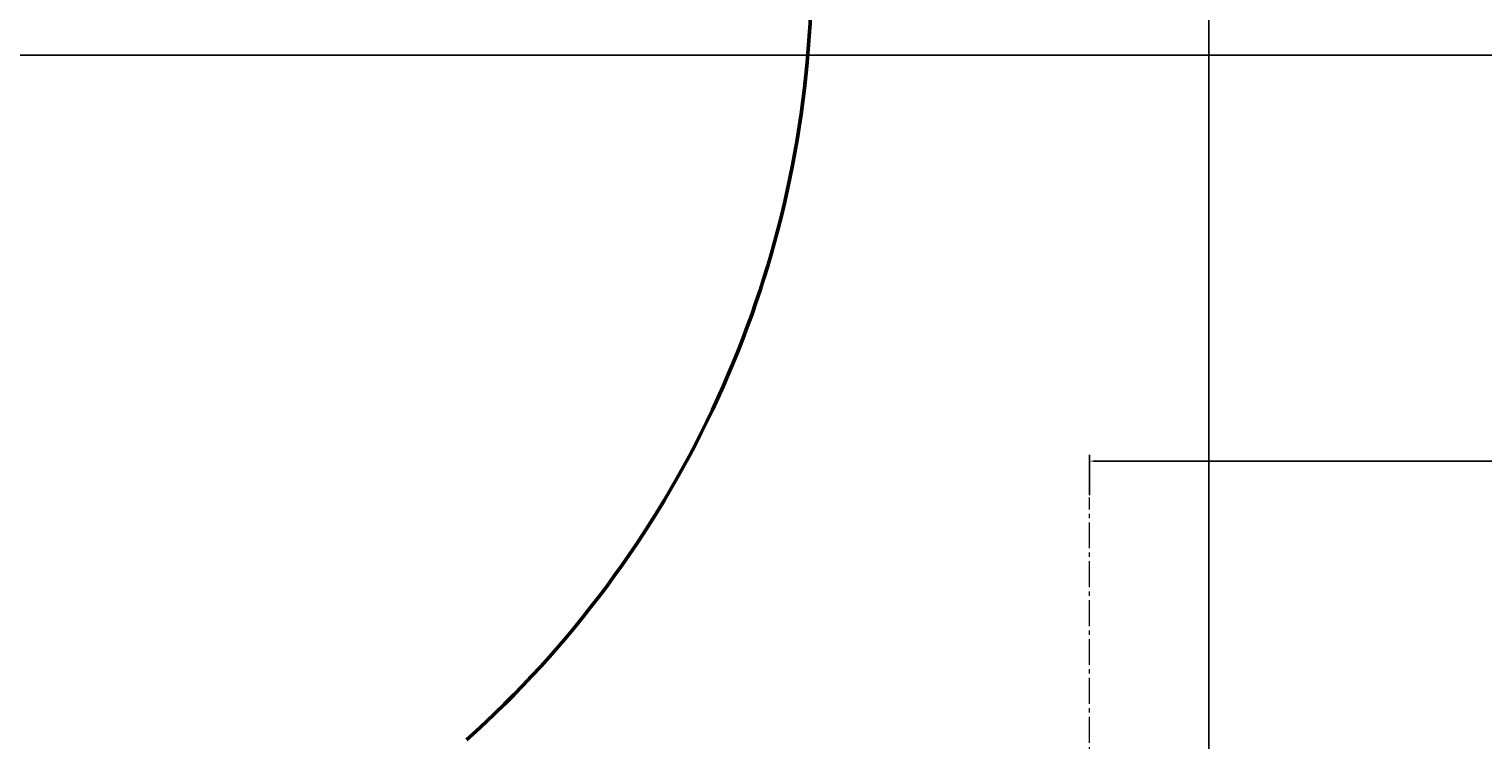
# Model space of a CAD drawing. Units: millimetres. Extents: x -60 to 113, y -37 to 126.
# Tile 7 of 17: x -23 to 19, y 27 to 48. Entities that reach past the tile are written whole.
import ezdxf

# ---------------------------------------------------------------- set-up
doc = ezdxf.new("R2010")
doc.units = ezdxf.units.MM
doc.header["$MEASUREMENT"] = 0
doc.linetypes.add('CENTER2', pattern=[1.125, 0.75, -0.125, 0.125, -0.125])
for name, color, linetype, lineweight in [('M-CNTR', 4, 'CENTER2', 18), ('M-DIMS', 2, 'Continuous', 25), ('M-OUTL', 7, 'Continuous', 50)]:
    doc.layers.add(name, color=color, linetype=linetype, lineweight=lineweight)
doc.styles.get("Standard").update_dxf_attribs({"font": 'arial.ttf'})
doc.dimstyles.get("Standard").update_dxf_attribs({"dimtxt": 0.18, "dimasz": 0.18, "dimexe": 0.18, "dimexo": 0.0625, "dimgap": 0.09, "dimtad": 0, "dimtih": 1, "dimtoh": 1, "dimdec": 4, "dimzin": 0, "dimdsep": 46, "dimtxsty": 'Standard', "dimcen": 0.09, "dimadec": 0, "dimazin": 0, "dimtfac": 1, "dimtdec": 4, "dimtofl": 0, "dimtmove": 0, "dimatfit": 3, "dimfxl": 1, "dimtolj": 1, "dimtzin": 0, "dimarcsym": 0})

# ---------------------------------------------------------------- blocks, each defined once
blk = doc.blocks.new('*U2')
at = {"layer": 'M-CNTR', "color": 0, "transparency": 16777216}
blk.add_line((0, 5.4), (0, 27.12), dxfattribs=at)
blk = doc.blocks.new('*D12')
at = {"layer": 'Defpoints', "color": 0, "transparency": 16777216}
for p in [(10.532, 88.533), (-58.719, 6.903), (11.329, 6.903)]:
    blk.add_point(p, dxfattribs=at)
at = {"layer": 'M-DIMS', "color": 0, "lineweight": -2, "transparency": 16777216}
for p, q in [((10.47, 88.533), (-58.899, 88.533)), ((-58.719, 88.353), (-58.719, 48.829)), ((-58.719, 7.083), (-58.719, 46.607)), ((11.267, 6.903), (-58.899, 6.903))]:
    blk.add_line(p, q, dxfattribs=at)
at = {"layer": 'M-DIMS', "color": 0, "transparency": 16777216}
for points in [[(-58.749, 88.353), (-58.689, 88.353), (-58.719, 88.533)], [(-58.749, 7.083), (-58.689, 7.083), (-58.719, 6.903)]]:
    blk.add_solid(points, dxfattribs=at)
at = {"layer": 'M-DIMS', "color": 0, "transparency": 16777216, "insert": (-58.719, 47.718), "char_height": 0.18, "attachment_point": 5}
blk.add_mtext('\\A1;{\\H11.11111x;82}', dxfattribs=at)
blk = doc.blocks.new('*D13')
at = {"layer": 'Defpoints', "color": 0, "transparency": 16777216}
for p in [(37.065, 46.813), (-39.303, 6.903), (7.267, 6.903)]:
    blk.add_point(p, dxfattribs=at)
at = {"layer": 'M-DIMS', "color": 0, "lineweight": -2, "transparency": 16777216}
for p, q in [((37.002, 46.813), (-39.483, 46.813)), ((-39.303, 46.633), (-39.303, 27.969)), ((-39.303, 7.083), (-39.303, 25.747)), ((7.204, 6.903), (-39.483, 6.903))]:
    blk.add_line(p, q, dxfattribs=at)
at = {"layer": 'M-DIMS', "color": 0, "transparency": 16777216}
for points in [[(-39.333, 46.633), (-39.273, 46.633), (-39.303, 46.813)], [(-39.333, 7.083), (-39.273, 7.083), (-39.303, 6.903)]]:
    blk.add_solid(points, dxfattribs=at)
at = {"layer": 'M-DIMS', "color": 0, "transparency": 16777216, "insert": (-39.303, 26.858), "char_height": 0.18, "attachment_point": 5}
blk.add_mtext('\\A1;{\\H11.11111x;40}', dxfattribs=at)
blk = doc.blocks.new('*D16')
at = {"layer": 'Defpoints', "color": 0, "transparency": 16777216}
for p in [(10.712, 88.533), (10.712, 88.533), (10.712, 6.442)]:
    blk.add_point(p, dxfattribs=at)
at = {"layer": 'M-DIMS', "color": 0, "lineweight": -2, "transparency": 16777216}
for p, q in [((10.712, 88.47), (10.712, 6.262)), ((10.712, 88.47), (10.712, 6.262)), ((10.532, 6.442), (10.352, 6.442)), ((10.892, 6.442), (11.072, 6.442))]:
    blk.add_line(p, q, dxfattribs=at)
at = {"layer": 'M-DIMS', "color": 0, "transparency": 16777216}
for points in [[(10.532, 6.472), (10.532, 6.412), (10.712, 6.442)], [(10.892, 6.472), (10.892, 6.412), (10.712, 6.442)]]:
    blk.add_solid(points, dxfattribs=at)
at = {"layer": 'M-DIMS', "color": 0, "transparency": 16777216, "insert": (11.536, 6.442), "char_height": 0.18, "attachment_point": 5}
blk.add_mtext('\\A1;0.0000', dxfattribs=at)
blk = doc.blocks.new('*D17')
at = {"layer": 'Defpoints', "color": 0, "transparency": 16777216}
for p in [(67.355, 124.823), (10.532, 88.533), (67.355, 6.442)]:
    blk.add_point(p, dxfattribs=at)
at = {"layer": 'M-DIMS', "color": 0, "lineweight": -2, "transparency": 16777216}
for p, q in [((10.532, 88.595), (10.532, 125.003)), ((67.355, 6.504), (67.355, 125.003)), ((10.712, 124.823), (37.422, 124.823)), ((67.175, 124.823), (40.465, 124.823))]:
    blk.add_line(p, q, dxfattribs=at)
at = {"layer": 'M-DIMS', "color": 0, "transparency": 16777216}
for points in [[(10.712, 124.853), (10.712, 124.793), (10.532, 124.823)], [(67.175, 124.853), (67.175, 124.793), (67.355, 124.823)]]:
    blk.add_solid(points, dxfattribs=at)
at = {"layer": 'M-DIMS', "color": 0, "transparency": 16777216, "insert": (38.944, 124.823), "char_height": 0.18, "attachment_point": 5}
blk.add_mtext('\\A1;{\\H11.11111x;56}', dxfattribs=at)
blk = doc.blocks.new('*D18')
at = {"layer": 'Defpoints', "color": 0, "transparency": 16777216}
for p in [(37.067, 35.073), (7.267, 34.023), (37.067, 33.992)]:
    blk.add_point(p, dxfattribs=at)
at = {"layer": 'M-DIMS', "color": 0, "lineweight": -2, "transparency": 16777216}
for p, q in [((7.267, 34.085), (7.267, 35.253)), ((7.447, 35.073), (20.648, 35.073)), ((36.887, 35.073), (23.685, 35.073)), ((37.067, 34.055), (37.067, 35.253))]:
    blk.add_line(p, q, dxfattribs=at)
at = {"layer": 'M-DIMS', "color": 0, "transparency": 16777216}
for points in [[(7.447, 35.103), (7.447, 35.043), (7.267, 35.073)], [(36.887, 35.103), (36.887, 35.043), (37.067, 35.073)]]:
    blk.add_solid(points, dxfattribs=at)
at = {"layer": 'M-DIMS', "color": 0, "transparency": 16777216, "insert": (22.167, 35.073), "char_height": 0.18, "attachment_point": 5}
blk.add_mtext('\\A1;{\\H11.11111x;30}', dxfattribs=at)

msp = doc.modelspace()

# ---------------------------------------------------------------- linework, layer by layer
at = {"layer": 'M-OUTL'}
msp.add_arc((-30.77517, 49.3506), 30, 311.866655, 43.425324, dxfattribs=at)

# ---------------------------------------------------------------- block references
at = {"layer": 'M-CNTR'}
msp.add_blockref('*U2', (7.26659, 6.9027), dxfattribs=at)

# ---------------------------------------------------------------- dimensions: what is measured, and where the dimension line sits
at = {"layer": 'M-DIMS'}
for base, p1, p2, text, picture, middle in [((67.35481, 124.82251), (10.53227, 88.53289), (67.35481, 6.44179), '{\\H11.11111x;56}', '*D17', (38.94354, 124.82251)), ((37.06673, 35.07294), (7.26659, 34.0227), (37.06673, 33.99249), '{\\H11.11111x;30}', '*D18', (22.16666, 35.07294))]:
    dim = msp.add_linear_dim(base=base, p1=p1, p2=p2, text=text, dimstyle='Standard', override={"dimclrd": 0, "dimclre": 0, "dimclrt": 0}, dxfattribs=at)
    dim.commit()
    dim.dimension.update_dxf_attribs({"geometry": picture, "text_midpoint": middle})
for base, p1, p2, text, picture, middle in [((-58.71857, 6.9027), (10.53227, 88.53289), (11.32938, 6.9027), '{\\H11.11111x;82}', '*D12', (-58.71857, 47.71779)), ((-39.30316, 6.9027), (37.06463, 46.81263), (7.26659, 6.9027), '{\\H11.11111x;40}', '*D13', (-39.30316, 26.85766))]:
    dim = msp.add_linear_dim(base=base, p1=p1, p2=p2, angle=90, text=text, dimstyle='Standard', override={"dimclrd": 0, "dimclre": 0, "dimclrt": 0}, dxfattribs=at)
    dim.commit()
    dim.dimension.update_dxf_attribs({"geometry": picture, "text_midpoint": middle})
dim = msp.add_linear_dim(base=(10.712269814, 6.441792179), p1=(10.712269814, 88.5328900903), p2=(10.712269814, 88.5328900903), dimstyle='Standard', override={"dimclrd": 0, "dimclre": 0, "dimclrt": 0}, dxfattribs=at)
dim.commit()
dim.dimension.update_dxf_attribs({"geometry": '*D16', "text_midpoint": (11.5355917785, 6.441792179)})

doc.saveas('drawing.dxf')
